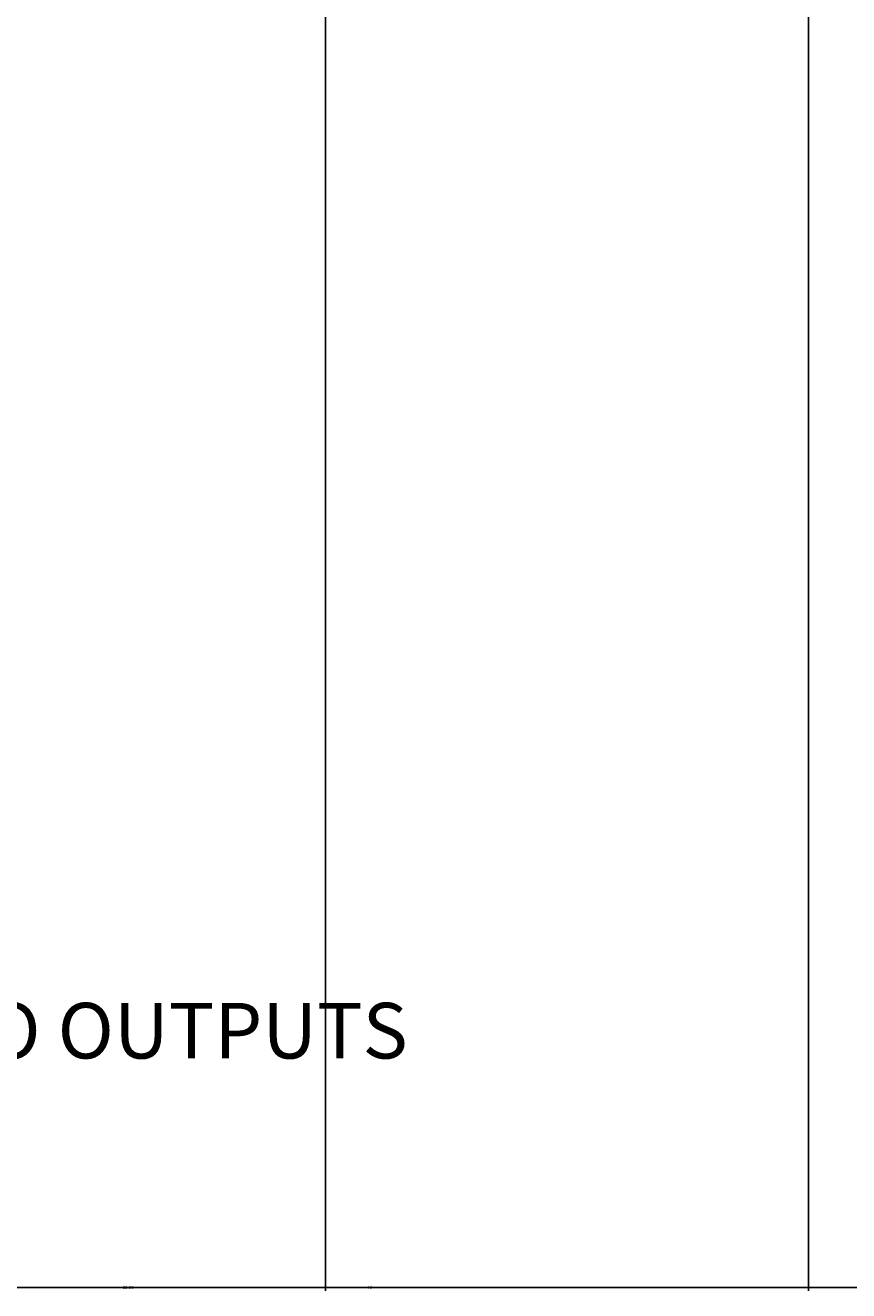
# Model space of a CAD drawing. Units: inches. Extents: x 738 to 1068, y 378 to 757.
# Tile 7 of 41: x 787 to 833, y 378 to 449. Entities that reach past the tile are written whole.
import ezdxf

# ---------------------------------------------------------------- set-up
doc = ezdxf.new("R2010")
doc.units = ezdxf.units.IN
doc.header["$MEASUREMENT"] = 0
doc.layers.add('A-ANNO-DIMS', color=2, linetype='Continuous', lineweight=18)
doc.layers.add('E-ANNO-TEXT', color=7, linetype='Continuous', lineweight=18)
doc.styles.get("Standard").update_dxf_attribs({"font": 'arial.ttf'})
doc.dimstyles.get("Standard").update_dxf_attribs({"dimtxt": 0.18, "dimasz": 0.18, "dimexe": 0.18, "dimexo": 0.0625, "dimgap": 0.09, "dimtad": 0, "dimtih": 1, "dimtoh": 1, "dimdec": 4, "dimzin": 0, "dimdsep": 46, "dimtxsty": 'Standard', "dimcen": 0.09, "dimadec": 0, "dimazin": 0, "dimtfac": 1, "dimtdec": 4, "dimtofl": 0, "dimtmove": 0, "dimatfit": 3, "dimfxl": 1, "dimtolj": 1, "dimtzin": 0, "dimarcsym": 0})

# ---------------------------------------------------------------- blocks, each defined once
blk = doc.blocks.new('*D17')
at = {"layer": 'A-ANNO-DIMS', "color": 0, "lineweight": -2, "transparency": 16777216}
for p, q in [((756.324, 415.842), (756.324, 378.239)), ((1050.049, 415.919), (1050.049, 378.239)), ((756.504, 378.419), (902.791, 378.419)), ((1049.869, 378.419), (903.582, 378.419))]:
    blk.add_line(p, q, dxfattribs=at)
at = {"layer": 'A-ANNO-DIMS', "color": 0, "transparency": 16777216}
for points in [[(756.504, 378.449), (756.504, 378.389), (756.324, 378.419)], [(1049.869, 378.449), (1049.869, 378.389), (1050.049, 378.419)]]:
    blk.add_solid(points, dxfattribs=at)
at = {"layer": 'Defpoints', "color": 0, "transparency": 16777216}
for p in [(756.324, 415.904), (1050.049, 415.982), (1050.049, 378.419)]:
    blk.add_point(p, dxfattribs=at)
at = {"layer": 'A-ANNO-DIMS', "color": 0, "transparency": 16777216, "insert": (903.186, 378.419), "char_height": 0.18, "attachment_point": 5}
blk.add_mtext('\\A1;293.7', dxfattribs=at)
blk = doc.blocks.new('*D25')
at = {"layer": 'A-ANNO-DIMS', "color": 0, "lineweight": -2, "transparency": 16777216}
for p, q in [((781.49, 646.923), (781.49, 378.239)), ((803.522, 646.923), (803.522, 378.239)), ((781.67, 378.419), (792.111, 378.419)), ((803.342, 378.419), (792.901, 378.419))]:
    blk.add_line(p, q, dxfattribs=at)
at = {"layer": 'A-ANNO-DIMS', "color": 0, "transparency": 16777216}
for points in [[(781.67, 378.449), (781.67, 378.389), (781.49, 378.419)], [(803.342, 378.449), (803.342, 378.389), (803.522, 378.419)]]:
    blk.add_solid(points, dxfattribs=at)
at = {"layer": 'Defpoints', "color": 0, "transparency": 16777216}
for p in [(781.49, 646.985), (803.522, 646.985), (803.522, 378.419)]:
    blk.add_point(p, dxfattribs=at)
at = {"layer": 'A-ANNO-DIMS', "color": 0, "transparency": 16777216, "insert": (792.506, 378.419), "char_height": 0.18, "attachment_point": 5}
blk.add_mtext('\\A1;22.03', dxfattribs=at)
blk = doc.blocks.new('*D34')
at = {"layer": 'A-ANNO-DIMS', "color": 0, "lineweight": -2, "transparency": 16777216}
for p, q in [((781.49, 686.266), (781.49, 378.239)), ((830.489, 686.266), (830.489, 378.239)), ((781.67, 378.419), (805.767, 378.419)), ((830.309, 378.419), (806.212, 378.419))]:
    blk.add_line(p, q, dxfattribs=at)
at = {"layer": 'A-ANNO-DIMS', "color": 0, "transparency": 16777216}
for points in [[(781.67, 378.449), (781.67, 378.389), (781.49, 378.419)], [(830.309, 378.449), (830.309, 378.389), (830.489, 378.419)]]:
    blk.add_solid(points, dxfattribs=at)
at = {"layer": 'Defpoints', "color": 0, "transparency": 16777216}
for p in [(781.49, 686.329), (830.489, 686.329), (830.489, 378.419)]:
    blk.add_point(p, dxfattribs=at)
at = {"layer": 'A-ANNO-DIMS', "color": 0, "transparency": 16777216, "insert": (805.99, 378.419), "char_height": 0.18, "attachment_point": 5}
blk.add_mtext('\\A1;49', dxfattribs=at)
blk = doc.blocks.new('*D38')
at = {"layer": 'A-ANNO-DIMS', "color": 0, "lineweight": -2, "transparency": 16777216}
for p, q in [((781.485, 593.017), (781.485, 378.239)), ((887.04, 593.067), (887.04, 378.239)), ((781.665, 378.419), (833.807, 378.419)), ((886.86, 378.419), (834.718, 378.419))]:
    blk.add_line(p, q, dxfattribs=at)
at = {"layer": 'A-ANNO-DIMS', "color": 0, "transparency": 16777216}
for points in [[(781.665, 378.449), (781.665, 378.389), (781.485, 378.419)], [(886.86, 378.449), (886.86, 378.389), (887.04, 378.419)]]:
    blk.add_solid(points, dxfattribs=at)
at = {"layer": 'Defpoints', "color": 0, "transparency": 16777216}
for p in [(781.485, 593.08), (887.04, 593.13), (887.04, 378.419)]:
    blk.add_point(p, dxfattribs=at)
at = {"layer": 'A-ANNO-DIMS', "color": 0, "transparency": 16777216, "insert": (834.263, 378.419), "char_height": 0.18, "attachment_point": 5}
blk.add_mtext('\\A1;105.56', dxfattribs=at)

msp = doc.modelspace()

# ---------------------------------------------------------------- texts
at = {"layer": 'E-ANNO-TEXT'}
msp.add_text('MCR2-2 TO OUTPUTS', height=3.107428, dxfattribs=at).set_placement((765.9672, 391.2068))

# ---------------------------------------------------------------- dimensions: what is measured, and where the dimension line sits
at = {"layer": 'A-ANNO-DIMS'}
for base, p1, p2, override, picture, middle in [((830.4893, 378.4191), (781.4897, 686.329), (830.4893, 686.329), {"dimdec": 0, "dimlfac": 1, "dimrnd": 0, "dimzin": 0, "dimdsep": 46, "dimlunit": 2}, '*D34', (805.9895, 378.4191)), ((803.5218, 378.4191), (781.4897, 646.9853), (803.5218, 646.9853), {"dimdec": 2, "dimlfac": 1, "dimrnd": 0, "dimzin": 0, "dimdsep": 46, "dimlunit": 2}, '*D25', (792.5057, 378.4191)), ((887.0404, 378.4191), (781.4846, 593.0796), (887.0404, 593.1296), {"dimdec": 2, "dimlfac": 1, "dimrnd": 0, "dimzin": 0, "dimdsep": 46, "dimlunit": 2}, '*D38', (834.2625, 378.4191)), ((1050.0492, 378.4191), (756.3236, 415.904), (1050.0492, 415.982), {"dimdec": 1, "dimlfac": 1, "dimrnd": 0, "dimzin": 0, "dimdsep": 46, "dimlunit": 2}, '*D17', (903.1864, 378.4191))]:
    dim = msp.add_linear_dim(base=base, p1=p1, p2=p2, dimstyle='Standard', override=override, dxfattribs=at)
    dim.commit()
    dim.dimension.update_dxf_attribs({"geometry": picture, "text_midpoint": middle})

doc.saveas('drawing.dxf')
